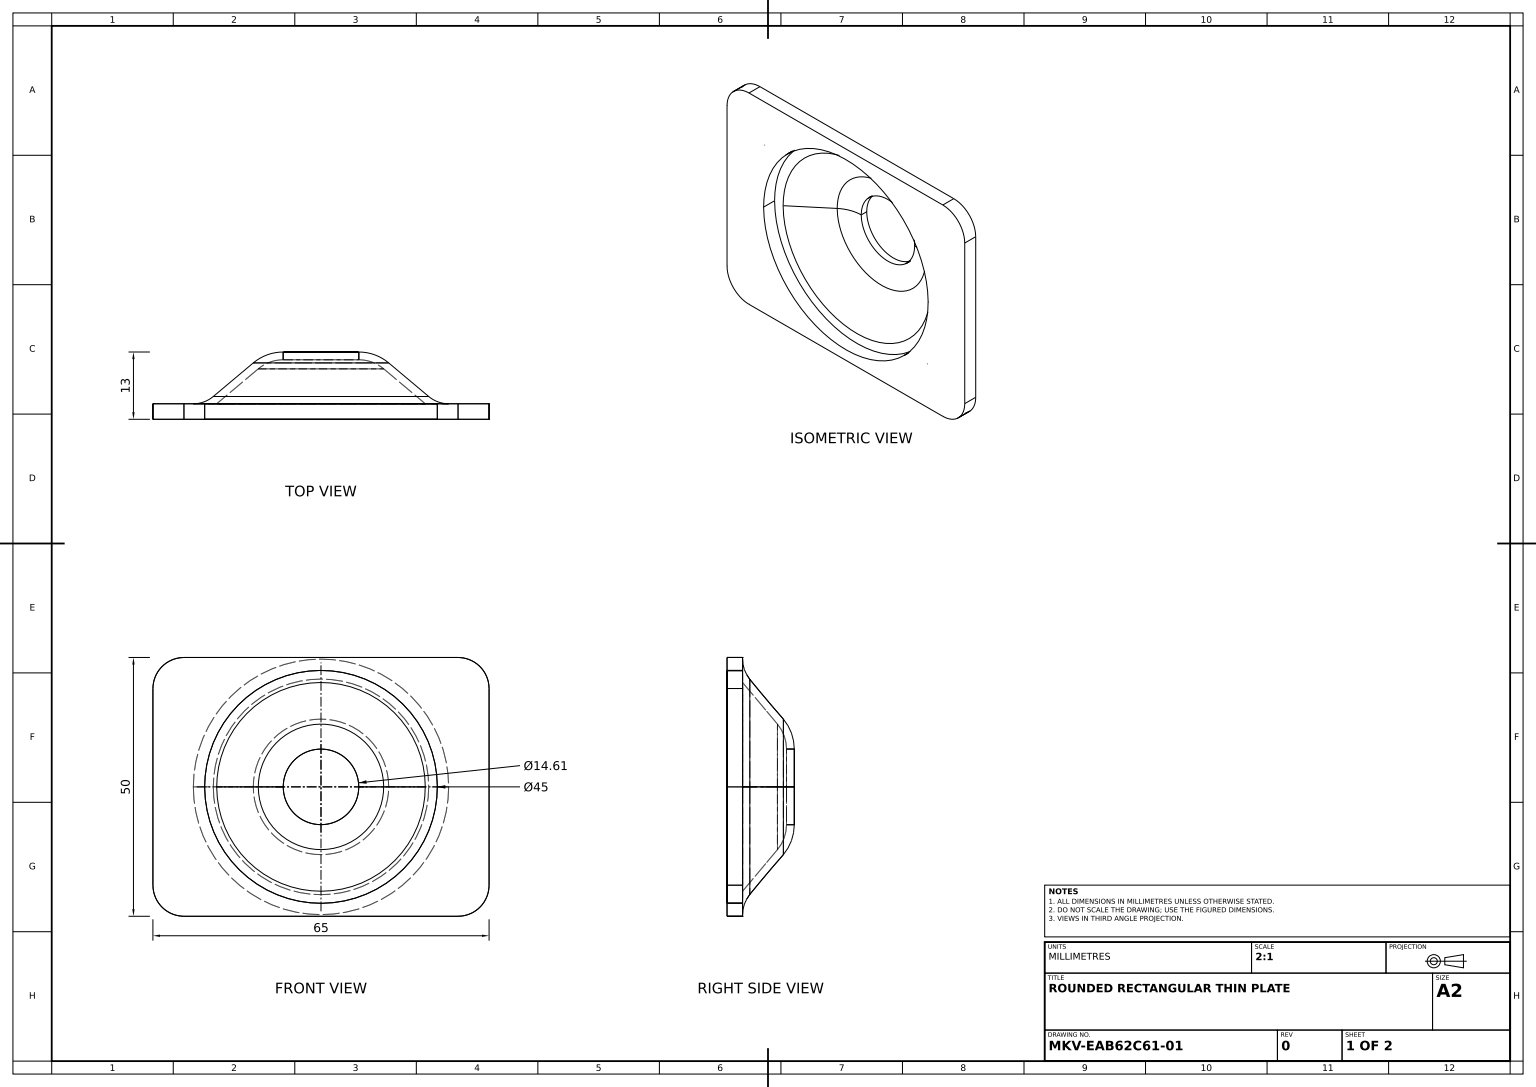
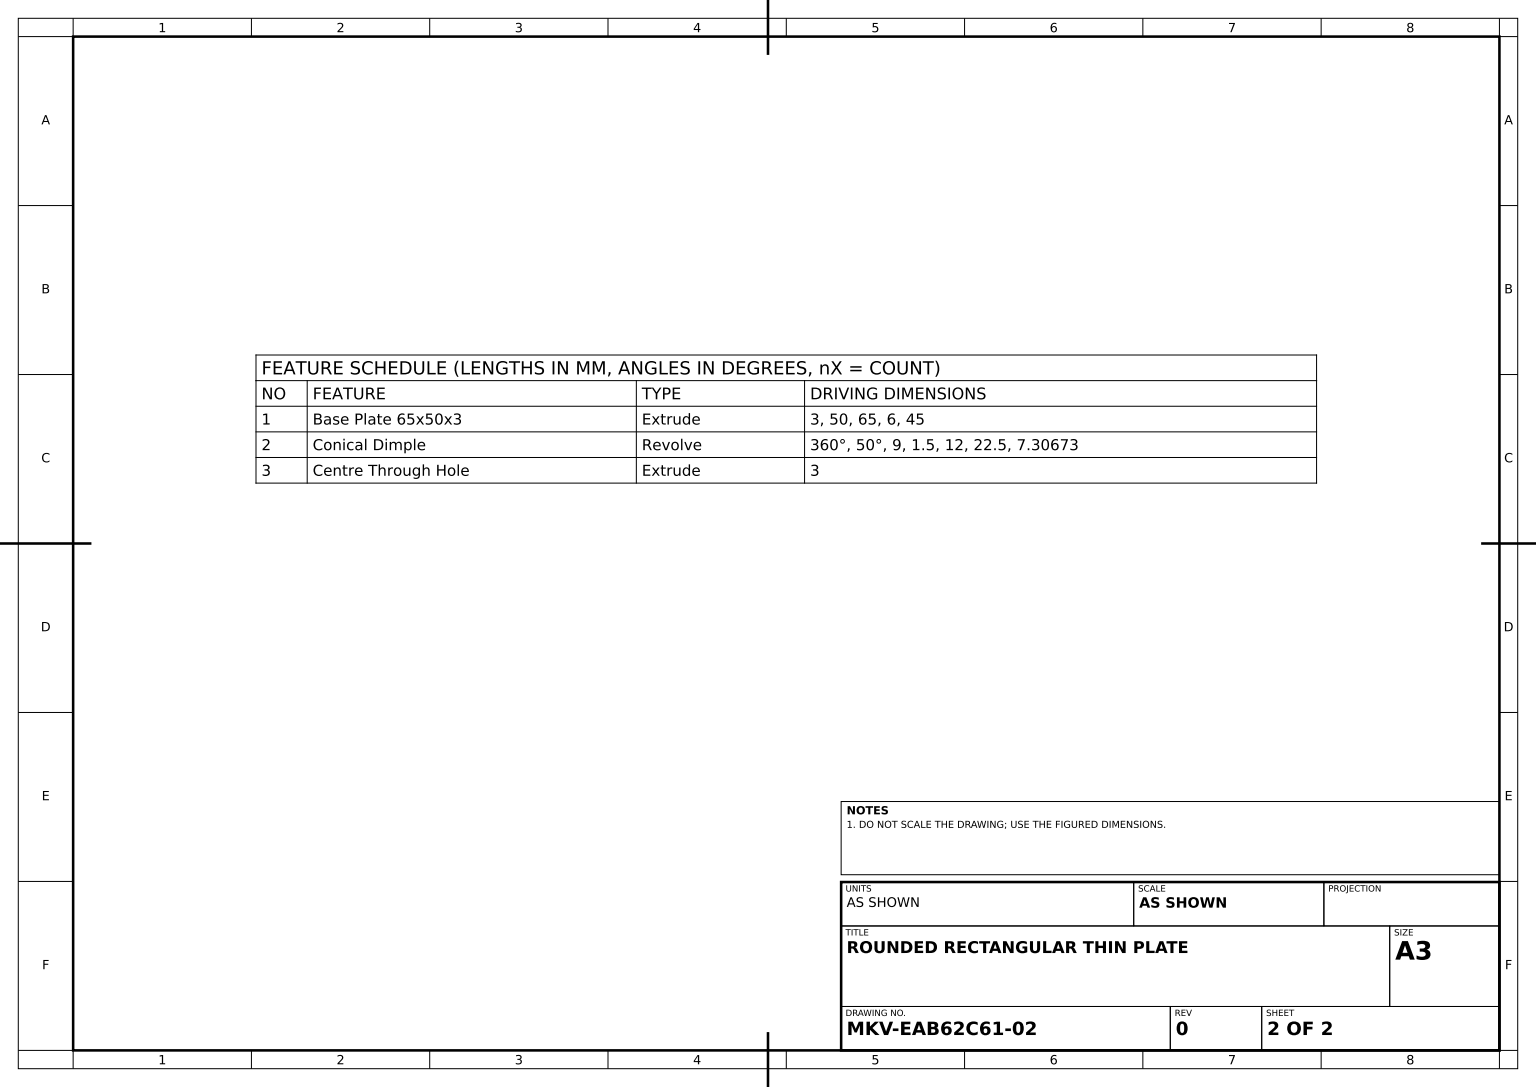
SolidWorks part; units mm, degrees
material "Plain Carbon Steel"
ref_plane "Front Plane" through (0, 0, 0) normal (0, 0, 1) x (1, 0, 0)
ref_plane "Top Plane" through (0, 0, 0) normal (0, 1, 0) x (1, 0, 0)
ref_plane "Right Plane" through (0, 0, 0) normal (1, 0, 0) x (0, 0, -1)
sketch "Plate Profile Sketch" plane through (0, 0, 0) normal (0, 0, 1) x (1, 0, 0)
  line L1 (-26.5, -25) -> (26.5, -25)
  line L2 (-32.5, -19) -> (-32.5, 19)
  line L3 (-26.5, 25) -> (26.5, 25)
  line L4 (32.5, -19) -> (32.5, 19)
  line L5 (-32.5, -25) -> (32.5, 25) construction
  line L6 (-32.5, 25) -> (32.5, -25) construction
  arc A0 (-26.5, -25) -> (-32.5, -19) centre (-26.5, -19) cw
  arc A1 (26.5, -25) -> (32.5, -19) centre (26.5, -19) ccw
  arc A2 (26.5, 25) -> (32.5, 19) centre (26.5, 19) cw
  arc A3 (-32.5, 19) -> (-26.5, 25) centre (-26.5, 19) cw
  circle A4 centre (0, 0) radius 22.5
  point P0 (0, 0)
  dimension "D3" = 6
  dimension "D4" = 45
  dimension "D1" = 50
  dimension "D2" = 65
extrude "Base Plate 65x50x3" add sketch "Plate Profile Sketch" along normal blind 3
sketch "Conical Dimple Profile Sketch" plane through (0, 0, 0) normal (0, 1, 0) x (1, 0, 0)
  line L0 (0, -5.7878) -> (0, 15.0386) construction
  line L1 (13.0918, 7.8944) -> (20.8271, 1.4037)
  line L2 (0, 10) -> (7.3067, 10)
  line L4 (24.6838, 0) -> (20.1664, 0)
  line L5 (0, 10) -> (0, 8.5)
  line L6 (20.1664, 0) -> (22.5, 0)
  line L7 (26.5, 0) -> (-26.5, 0) construction
  line L9 (0, 8.5) -> (7.3067, 8.5)
  line L10 (12.1276, 6.7453) -> (20.1664, 0)
  line L13 (1.5, 8.5) -> (7.3067, 8.5) construction
  line L14 (13.0918, 7.8944) -> (22.5, 0) construction
  line L15 (1.5, 1.5) -> (18.3788, 1.5) construction
  line L16 (1.5, 8.5) -> (1.5, 1.5) construction
  line L17 (12.1276, 6.7453) -> (18.3788, 1.5) construction
  line L19 (0, 10) -> (0, 0) construction
  line L20 (0, 0) -> (22.5, 0) construction
  arc A0 (7.3067, 10) -> (13.0918, 7.8944) centre (7.3067, 1) cw
  arc A1 (7.3067, 8.5) -> (12.1276, 6.7453) centre (7.3067, 1) cw
  arc A2 (20.8271, 1.4037) -> (24.6838, 0) centre (24.6838, 6) ccw
  dimension "D4" = 9
  dimension "D6" = 12
  dimension "D1" = 50
  dimension "D2" = 7.3067
  dimension "D3" = 22.5
  dimension "D5" = 1.5
revolve "Conical Dimple" add sketch "Conical Dimple Profile Sketch" angle 360 about L0
sketch "Centre Hole Sketch" plane through (0, 0, -10) normal (0, 0, -1) x (-1, 0, 0)
  circle A1 centre (0, 0) radius 7.3067
  circle A2 centre (0, 0) radius 7.3067
  dimension "D1" = 0
extrude "Centre Through Hole" cut sketch "Centre Hole Sketch" against normal blind 3
